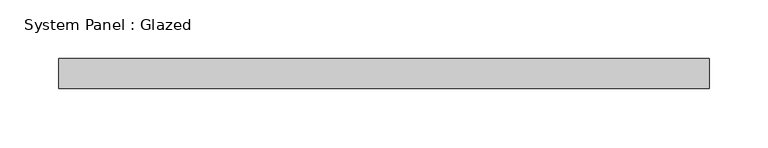
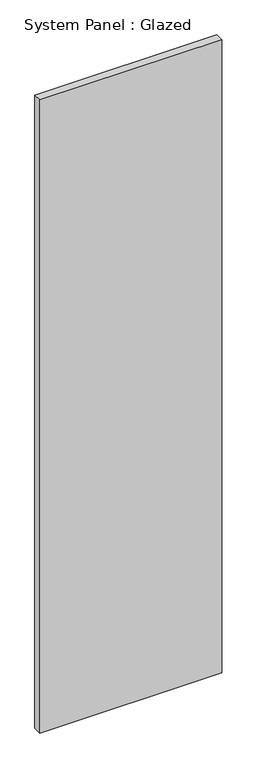
"""IFC4 building model written with IfcOpenShell, lengths in millimetres: plate geometry, System Panel : Glazed."""

from ifc_helpers import new_model, si_unit, origin, origin_with_axes, place, context, project, spatial, polyline, outline, extrude, source, transform, mapped, element, save


def system_panel_glazed_a8841a5f(model_context):
    return source(origin(), model_context, "Body", "SweptSolid", [
        extrude(outline(polyline([(276.225, 19.05), (-276.225, 19.05), (-276.225, 44.45), (276.225, 44.45), (276.225, 19.05)])), origin_with_axes(), (0.0, 0.0, 1.0), 2032.0),
    ])


if __name__ == "__main__":
    model = new_model("IFC4")
    model_context = context("Model", 3, world=origin())
    ifc_project = project(units=[si_unit("LENGTHUNIT", "METRE", prefix="MILLI")], contexts=[model_context])
    site = spatial("IfcSite", under=ifc_project)
    building = spatial("IfcBuilding", under=site)
    placement = place(None, origin())
    system_panel_glazed_shape = system_panel_glazed_a8841a5f(model_context)
    element("IfcPlate", 1, ObjectType="System Panel : Glazed", at=placement, inside=building, context=model_context, shape_type="MappedRepresentation", body=[
        mapped(system_panel_glazed_shape, transform((0.0, 0.0, 0.0), x_axis=(1.0, 0.0, 0.0), y_axis=(0.0, 1.0, 0.0), z_axis=(0.0, 0.0, 1.0))),
    ])
    save(model, "model.ifc")

# Revit data of these elements
# Type "System Panel : Glazed"
#   Construction Type Id = "GSP4R"
#   Analytic Construction = "1/8 in Pilkington single glazing"
#   Visual Light Transmittance = 0.9
#   Solar Heat Gain Coefficient = 0.86
#   Heat Transfer Coefficient (U) = 1.18115 BTU/(h·ft²·°F)
#   Define Thermal Properties by = 1
# Element 1 (IfcPlate, "System Panel : Glazed")
#   Materials on its faces: "Glass"
# Materials
#   "Glass": class "Glass", colour RGB 0 128 192, transparency 0.75, Description = "Soda Lime Glass", Cost = 0
